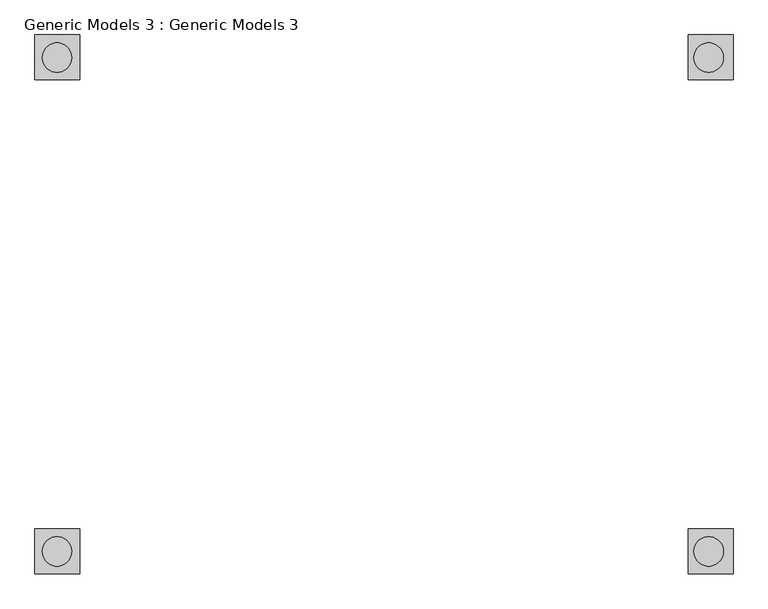
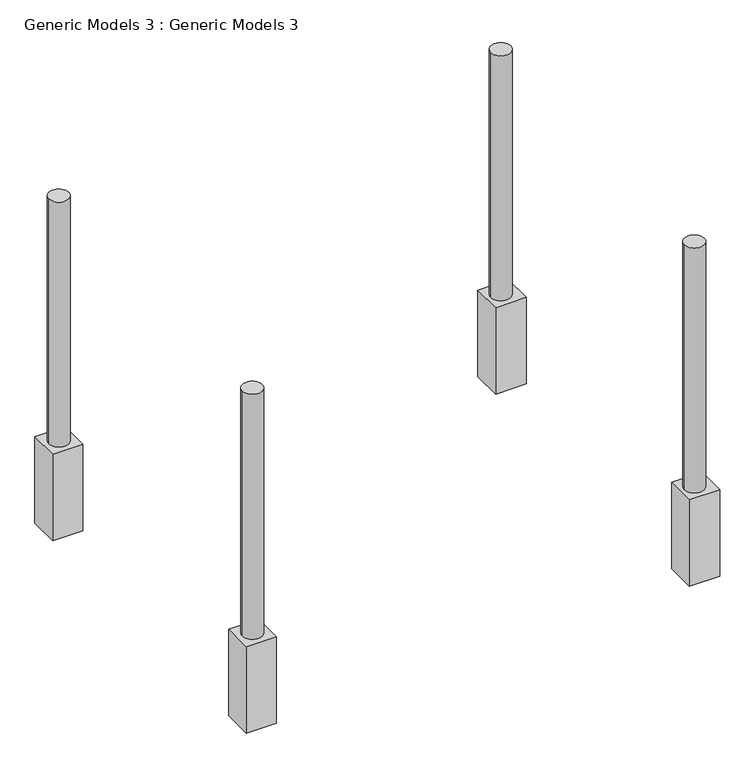
"""IFC4 building model written with IfcOpenShell, lengths in millimetres: proxy geometry, Generic Models 3 : Generic Models 3."""

from ifc_helpers import new_model, si_unit, point, frame, frame_2d, origin, place, context, project, spatial, polyline, circle_curve, trimmed, segment, composite_curve, outline, extrude, source, transform, mapped, element, save


def generic_models_3_generic_models_3_02764364(model_context):
    return source(origin(), model_context, "Body", "SweptSolid", [
        extrude(outline(composite_curve([segment(trimmed(circle_curve(frame_2d((-15069.5685174, 3341.4773079)), 99.7350324), [point((-15169.3035498, 3341.4773079))], [point((-14969.8334849, 3341.4773079))], False, "CARTESIAN"), True, "CONTINUOUS"), segment(trimmed(circle_curve(frame_2d((-15069.5685174, 3341.4773079)), 99.7350324), [point((-14969.8334849, 3341.4773079))], [point((-15169.3035498, 3341.4773079))], False, "CARTESIAN"), True, "CONTINUOUS")], self_intersect=False)), frame((0.0, 0.0, 304.8), z_axis=(0.0, 0.0, 1.0), x_axis=(1.0, 0.0, 0.0)), (0.0, 0.0, 1.0), 2590.8),
        extrude(outline(composite_curve([segment(trimmed(circle_curve(frame_2d((-10649.9685174, 3341.4773079)), 99.7350324), [point((-10749.7035498, 3341.4773079))], [point((-10550.2334849, 3341.4773079))], False, "CARTESIAN"), True, "CONTINUOUS"), segment(trimmed(circle_curve(frame_2d((-10649.9685174, 3341.4773079)), 99.7350324), [point((-10550.2334849, 3341.4773079))], [point((-10749.7035498, 3341.4773079))], False, "CARTESIAN"), True, "CONTINUOUS")], self_intersect=False)), frame((0.0, 0.0, 304.8), z_axis=(0.0, 0.0, 1.0), x_axis=(1.0, 0.0, 0.0)), (0.0, 0.0, 1.0), 2590.8),
        extrude(outline(composite_curve([segment(trimmed(circle_curve(frame_2d((-10649.9685174, -11.3226921)), 99.7350324), [point((-10749.7035498, -11.3226921))], [point((-10550.2334849, -11.3226921))], False, "CARTESIAN"), True, "CONTINUOUS"), segment(trimmed(circle_curve(frame_2d((-10649.9685174, -11.3226921)), 99.7350324), [point((-10550.2334849, -11.3226921))], [point((-10749.7035498, -11.3226921))], False, "CARTESIAN"), True, "CONTINUOUS")], self_intersect=False)), frame((0.0, 0.0, 304.8), z_axis=(0.0, 0.0, 1.0), x_axis=(1.0, 0.0, 0.0)), (0.0, 0.0, 1.0), 2590.8),
        extrude(outline(composite_curve([segment(trimmed(circle_curve(frame_2d((-15069.5685174, -11.3226921)), 99.7350324), [point((-15169.3035498, -11.3226921))], [point((-14969.8334849, -11.3226921))], False, "CARTESIAN"), True, "CONTINUOUS"), segment(trimmed(circle_curve(frame_2d((-15069.5685174, -11.3226921)), 99.7350324), [point((-14969.8334849, -11.3226921))], [point((-15169.3035498, -11.3226921))], False, "CARTESIAN"), True, "CONTINUOUS")], self_intersect=False)), frame((0.0, 0.0, 304.8), z_axis=(0.0, 0.0, 1.0), x_axis=(1.0, 0.0, 0.0)), (0.0, 0.0, 1.0), 2590.8),
        extrude(outline(polyline([(-14916.206326, 141.3173763), (-14916.206326, -163.942926), (-15219.4827503, -163.942926), (-15219.4827503, 141.3173763), (-14916.206326, 141.3173763)])), frame((0.0, 0.0, -609.6), z_axis=(0.0, 0.0, 1.0), x_axis=(1.0, 0.0, 0.0)), (0.0, 0.0, 1.0), 914.4),
        extrude(outline(polyline([(-10483.9803096, 141.3173763), (-10483.9803096, -163.942926), (-10789.2406119, -163.942926), (-10789.2406119, 141.3173763), (-10483.9803096, 141.3173763)])), frame((0.0, 0.0, -609.6), z_axis=(0.0, 0.0, 1.0), x_axis=(1.0, 0.0, 0.0)), (0.0, 0.0, 1.0), 914.4),
        extrude(outline(polyline([(-10483.9803096, 3495.212945), (-10483.9803096, 3189.9526427), (-10789.2406119, 3189.9526427), (-10789.2406119, 3495.212945), (-10483.9803096, 3495.212945)])), frame((0.0, 0.0, -609.6), z_axis=(0.0, 0.0, 1.0), x_axis=(1.0, 0.0, 0.0)), (0.0, 0.0, 1.0), 914.4),
        extrude(outline(polyline([(-15219.4827503, 3189.9526427), (-15219.4827503, 3495.212945), (-14916.206326, 3495.212945), (-14916.206326, 3189.9526427), (-15219.4827503, 3189.9526427)])), frame((0.0, 0.0, -609.6), z_axis=(0.0, 0.0, 1.0), x_axis=(1.0, 0.0, 0.0)), (0.0, 0.0, 1.0), 914.4),
    ])


if __name__ == "__main__":
    model = new_model("IFC4")
    model_context = context("Model", 3, world=origin())
    ifc_project = project(units=[si_unit("LENGTHUNIT", "METRE", prefix="MILLI")], contexts=[model_context])
    site = spatial("IfcSite", under=ifc_project)
    building = spatial("IfcBuilding", under=site)
    placement = place(None, origin())
    generic_models_3_generic_models_3_shape = generic_models_3_generic_models_3_02764364(model_context)
    element("IfcBuildingElementProxy", 1, Name="Generic Models 3 : Generic Models 3", ObjectType="Generic Models 3 : Generic Models 3", at=placement, inside=building, context=model_context, shape_type="MappedRepresentation", body=[
        mapped(generic_models_3_generic_models_3_shape, transform((0.0, 0.0, 0.0), x_axis=(1.0, 0.0, 0.0), y_axis=(0.0, 1.0, 0.0), z_axis=(0.0, 0.0, 1.0))),
    ])
    save(model, "model.ifc")
